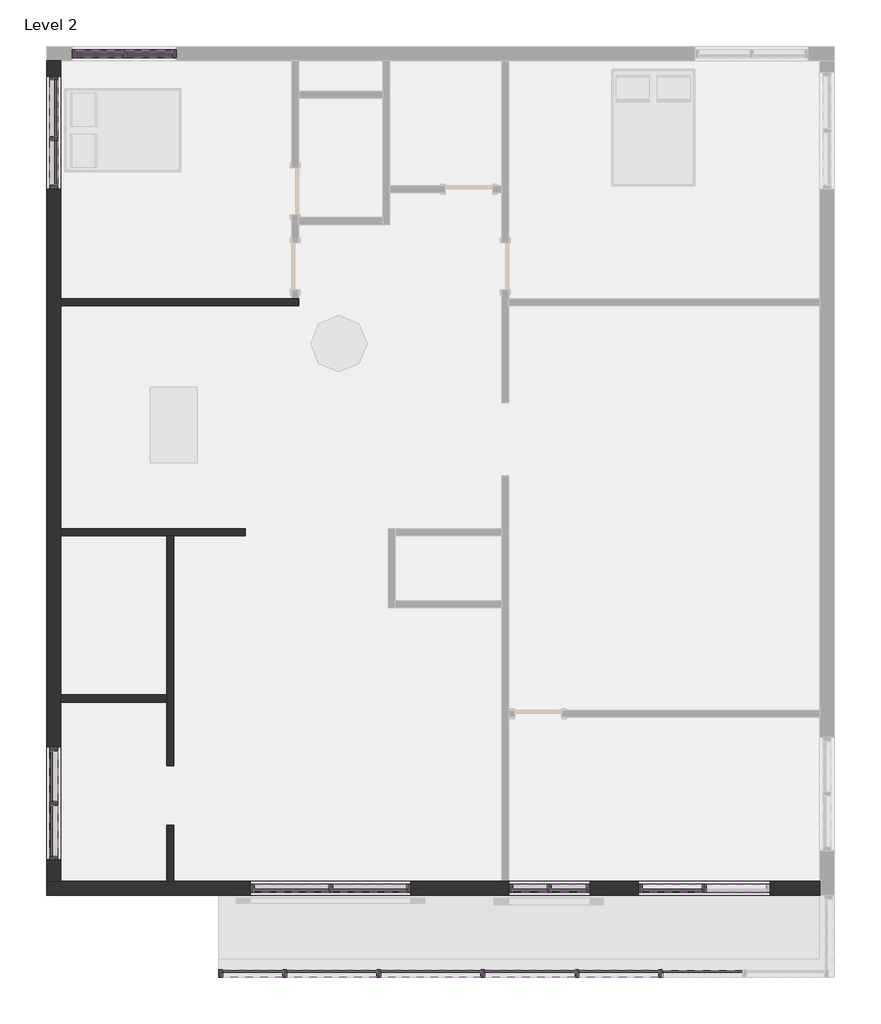
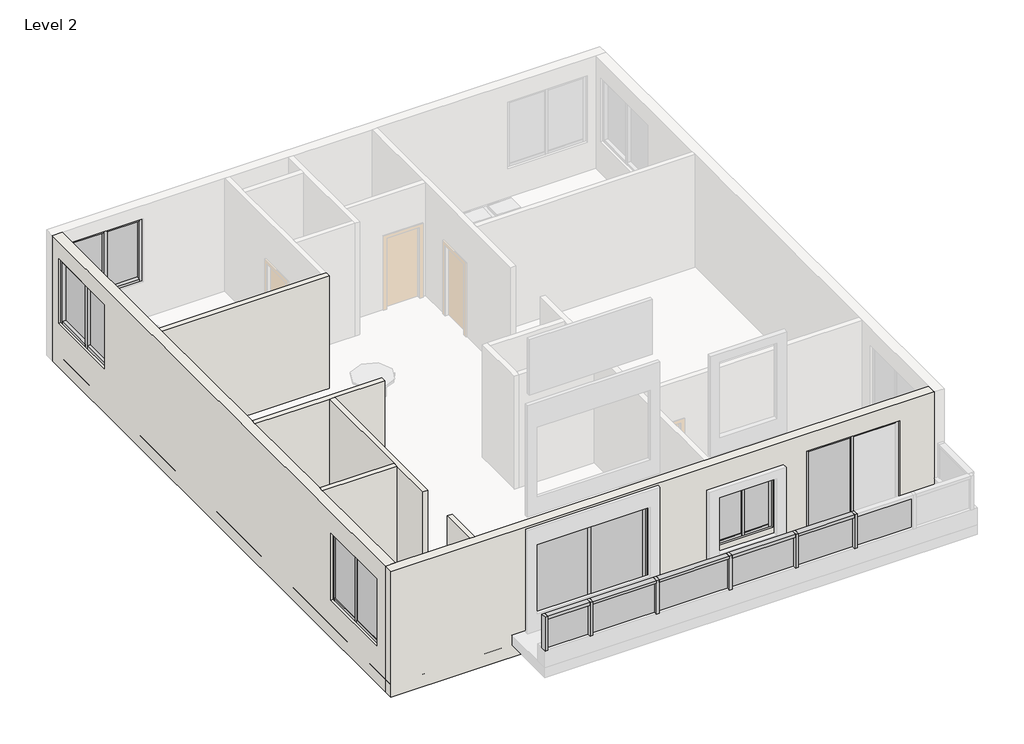
# One storey, part 1 of 2: 50 members, 17 plates, 7 walls.
"""IFC4 building model written with IfcOpenShell, lengths in millimetres."""

from ifc_helpers import new_model, si_unit, frame, origin, place, context, project, spatial, polyline, outline, extrude, faceted_brep, transform, mapped, element, save
from components import member_c17f1be2, member_3a0a7659, member_bb9b20bf, member_f3ef6fbd, member_e04b046a, member_80dcf73b, member_7007ad49, member_ff82125d, member_0ab19f0c, member_973bd760, member_801a2072, member_8e397d51, member_8dd6731c, member_87553b7f, member_e9c7f4a4, member_3112dcca, member_8a344535, member_99d3517c, member_dae9f1c3, member_4a1dde21, member_f7075cef, member_bf3bc0fd, member_d7462ea5, member_8ac64e86, system_panel_glazed_b08c4d22, system_panel_glazed_affe7bbf, system_panel_glazed_9eaa7c8f, system_panel_glazed_b4a21602, system_panel_glazed_4e5a3e53, system_panel_glazed_c585f582, system_panel_glazed_a27b9eb0, system_panel_glazed_060269ed, system_panel_glazed_0d05c03e, system_panel_glazed_4dc74c46, system_panel_glazed_e22b6634

model = new_model("IFC4")

# Units and contexts
model_context = context("Model", 3, world=origin())
ifc_project = project(units=[si_unit("LENGTHUNIT", "METRE", prefix="MILLI")], contexts=[model_context])

# Site, building, storey
site = spatial("IfcSite", under=ifc_project)
building = spatial("IfcBuilding", under=site)
storey = spatial("IfcBuildingStorey", under=building, Name="Level 2", Elevation=3048.0)

# Members
placement = place(None, origin())
member_shape = member_c17f1be2(model_context)
element("IfcMember", 1, ObjectType="Rectangular Mullion : 2.5\" x 5\" rectangular", at=placement, inside=storey, context=model_context, shape_type="MappedRepresentation", body=[
    mapped(member_shape, transform((-18883.3195233, -12680.6252569, 5586.6479842), x_axis=(0.0, 0.0, 1.0), y_axis=(1.0, 0.0, 0.0), z_axis=(0.0, 1.0, 0.0))),
])
element("IfcMember", 2, ObjectType="Rectangular Mullion : 2.5\" x 5\" rectangular", at=placement, inside=storey, context=model_context, shape_type="MappedRepresentation", body=[
    mapped(member_shape, transform((-18883.3195233, -11797.9752569, 5586.6479842), x_axis=(0.0, 0.0, 1.0), y_axis=(1.0, 0.0, 0.0), z_axis=(0.0, 1.0, 0.0))),
])
element("IfcMember", 3, ObjectType="Rectangular Mullion : 2.5\" x 5\" rectangular", at=placement, inside=storey, context=model_context, shape_type="MappedRepresentation", body=[
    mapped(member_shape, transform((-18883.3195233, -12617.1252569, 3956.7332675), x_axis=(0.0, 0.0, -1.0), y_axis=(1.0, 0.0, 0.0), z_axis=(0.0, -1.0, 0.0))),
])
element("IfcMember", 4, ObjectType="Rectangular Mullion : 2.5\" x 5\" rectangular", at=placement, inside=storey, context=model_context, shape_type="MappedRepresentation", body=[
    mapped(member_shape, transform((-18883.3195233, -13499.7752569, 3956.7332675), x_axis=(0.0, 0.0, -1.0), y_axis=(1.0, 0.0, 0.0), z_axis=(0.0, -1.0, 0.0))),
])
member_2_shape = member_3a0a7659(model_context)
element("IfcMember", 5, ObjectType="Rectangular Mullion : 2.5\" x 5\" rectangular", at=placement, inside=storey, context=model_context, shape_type="MappedRepresentation", body=[
    mapped(member_2_shape, transform((-17772.0695233, -533.0752569, 5767.2358325), x_axis=(0.0, 0.0, 1.0), y_axis=(0.0, -1.0, 0.0), z_axis=(1.0, 0.0, 0.0))),
])
element("IfcMember", 6, ObjectType="Rectangular Mullion : 2.5\" x 5\" rectangular", at=placement, inside=storey, context=model_context, shape_type="MappedRepresentation", body=[
    mapped(member_2_shape, transform((-16965.6195233, -533.0752569, 5767.2358325), x_axis=(0.0, 0.0, 1.0), y_axis=(0.0, -1.0, 0.0), z_axis=(1.0, 0.0, 0.0))),
])
element("IfcMember", 7, ObjectType="Rectangular Mullion : 2.5\" x 5\" rectangular", at=placement, inside=storey, context=model_context, shape_type="MappedRepresentation", body=[
    mapped(member_2_shape, transform((-17708.5695233, -533.0752569, 4232.1728983), x_axis=(0.0, 0.0, -1.0), y_axis=(0.0, -1.0, 0.0), z_axis=(-1.0, 0.0, 0.0))),
])
element("IfcMember", 8, ObjectType="Rectangular Mullion : 2.5\" x 5\" rectangular", at=placement, inside=storey, context=model_context, shape_type="MappedRepresentation", body=[
    mapped(member_2_shape, transform((-18515.0195233, -533.0752569, 4232.1728983), x_axis=(0.0, 0.0, -1.0), y_axis=(0.0, -1.0, 0.0), z_axis=(-1.0, 0.0, 0.0))),
])
member_3_shape = member_bb9b20bf(model_context)
element("IfcMember", 9, ObjectType="Rectangular Mullion : 2.5\" x 5\" rectangular", at=placement, inside=storey, context=model_context, shape_type="MappedRepresentation", body=[
    mapped(member_3_shape, transform((-17740.3195233, -533.0752569, 4232.1728983), x_axis=(1.0, 0.0, 0.0), y_axis=(0.0, -1.0, 0.0), z_axis=(0.0, 0.0, -1.0))),
])
member_4_shape = member_f3ef6fbd(model_context)
element("IfcMember", 10, ObjectType="Rectangular Mullion : 2.5\" x 5\" rectangular", at=placement, inside=storey, context=model_context, shape_type="MappedRepresentation", body=[
    mapped(member_4_shape, transform((-18578.5195233, -533.0752569, 5767.2358325), x_axis=(-1.0, 0.0, 0.0), y_axis=(0.0, -1.0, 0.0), z_axis=(0.0, 0.0, 1.0))),
])
element("IfcMember", 11, ObjectType="Rectangular Mullion : 2.5\" x 5\" rectangular", at=placement, inside=storey, context=model_context, shape_type="MappedRepresentation", body=[
    mapped(member_4_shape, transform((-16902.1195233, -533.0752569, 4232.1728983), x_axis=(1.0, 0.0, 0.0), y_axis=(0.0, -1.0, 0.0), z_axis=(0.0, 0.0, -1.0))),
])
member_5_shape = member_e04b046a(model_context)
element("IfcMember", 12, ObjectType="Rectangular Mullion : 2.5\" x 5\" rectangular", at=placement, inside=storey, context=model_context, shape_type="MappedRepresentation", body=[
    mapped(member_5_shape, transform((-18883.3195233, -12648.8752569, 3956.7332675), x_axis=(0.0, 1.0, 0.0), y_axis=(1.0, 0.0, 0.0), z_axis=(0.0, 0.0, -1.0))),
])
member_6_shape = member_80dcf73b(model_context)
element("IfcMember", 13, ObjectType="Rectangular Mullion : 2.5\" x 5\" rectangular", at=placement, inside=storey, context=model_context, shape_type="MappedRepresentation", body=[
    mapped(member_6_shape, transform((-18883.3195233, -13563.2752569, 5586.6479842), x_axis=(0.0, -1.0, 0.0), y_axis=(1.0, 0.0, 0.0), z_axis=(0.0, 0.0, 1.0))),
])
element("IfcMember", 14, ObjectType="Rectangular Mullion : 2.5\" x 5\" rectangular", at=placement, inside=storey, context=model_context, shape_type="MappedRepresentation", body=[
    mapped(member_6_shape, transform((-18883.3195233, -11734.4752569, 3956.7332675), x_axis=(0.0, 1.0, 0.0), y_axis=(1.0, 0.0, 0.0), z_axis=(0.0, 0.0, -1.0))),
])
member_7_shape = member_7007ad49(model_context)
element("IfcMember", 15, ObjectType="Rectangular Mullion : 2.5\" x 5\" rectangular", at=placement, inside=storey, context=model_context, shape_type="MappedRepresentation", body=[
    mapped(member_7_shape, transform((-18883.3195233, -2660.3252569, 5675.9534483), x_axis=(0.0, 0.0, 1.0), y_axis=(-1.0, 0.0, 0.0), z_axis=(0.0, -1.0, 0.0))),
])
member_8_shape = member_ff82125d(model_context)
element("IfcMember", 16, ObjectType="Rectangular Mullion : 2.5\" x 5\" rectangular", at=placement, inside=storey, context=model_context, shape_type="MappedRepresentation", body=[
    mapped(member_8_shape, transform((-18883.3195233, -1879.2752569, 5675.9534483), x_axis=(0.0, 0.0, 1.0), y_axis=(-1.0, 0.0, 0.0), z_axis=(0.0, -1.0, 0.0))),
])
member_9_shape = member_0ab19f0c(model_context)
element("IfcMember", 17, ObjectType="Rectangular Mullion : 2.5\" x 5\" rectangular", at=placement, inside=storey, context=model_context, shape_type="MappedRepresentation", body=[
    mapped(member_9_shape, transform((-18883.3195233, -1911.0252569, 4115.0021153), x_axis=(0.0, -1.0, 0.0), y_axis=(-1.0, 0.0, 0.0), z_axis=(0.0, 0.0, -1.0))),
])
element("IfcMember", 18, ObjectType="Rectangular Mullion : 2.5\" x 5\" rectangular", at=placement, inside=storey, context=model_context, shape_type="MappedRepresentation", body=[
    mapped(member_7_shape, transform((-18883.3195233, -1942.7752569, 4115.0021153), x_axis=(0.0, 0.0, -1.0), y_axis=(-1.0, 0.0, 0.0), z_axis=(0.0, 1.0, 0.0))),
])
element("IfcMember", 19, ObjectType="Rectangular Mullion : 2.5\" x 5\" rectangular", at=placement, inside=storey, context=model_context, shape_type="MappedRepresentation", body=[
    mapped(member_8_shape, transform((-18883.3195233, -958.5252569, 4115.0021153), x_axis=(0.0, 0.0, -1.0), y_axis=(-1.0, 0.0, 0.0), z_axis=(0.0, 1.0, 0.0))),
])
member_10_shape = member_973bd760(model_context)
element("IfcMember", 20, ObjectType="Rectangular Mullion : 2.5\" x 5\" rectangular", at=placement, inside=storey, context=model_context, shape_type="MappedRepresentation", body=[
    mapped(member_10_shape, transform((-18883.3195233, -2723.8252569, 4115.0021153), x_axis=(0.0, -1.0, 0.0), y_axis=(-1.0, 0.0, 0.0), z_axis=(0.0, 0.0, -1.0))),
])
element("IfcMember", 21, ObjectType="Rectangular Mullion : 2.5\" x 5\" rectangular", at=placement, inside=storey, context=model_context, shape_type="MappedRepresentation", body=[
    mapped(member_10_shape, transform((-18883.3195233, -895.0252569, 5675.9534483), x_axis=(0.0, 1.0, 0.0), y_axis=(-1.0, 0.0, 0.0), z_axis=(0.0, 0.0, 1.0))),
])
member_11_shape = member_801a2072(model_context)
element("IfcMember", 22, ObjectType="Rectangular Mullion : 2.5\" x 5\" rectangular", at=placement, inside=storey, context=model_context, shape_type="MappedRepresentation", body=[
    mapped(member_11_shape, transform((-8335.9695233, -14020.4752569, 5682.139627), x_axis=(0.0, 0.0, 1.0), y_axis=(0.0, 1.0, 0.0), z_axis=(-1.0, 0.0, 0.0))),
])
element("IfcMember", 23, ObjectType="Rectangular Mullion : 2.5\" x 5\" rectangular", at=placement, inside=storey, context=model_context, shape_type="MappedRepresentation", body=[
    mapped(member_11_shape, transform((-9371.0195233, -14020.4752569, 5682.139627), x_axis=(0.0, 0.0, 1.0), y_axis=(0.0, 1.0, 0.0), z_axis=(-1.0, 0.0, 0.0))),
])
element("IfcMember", 24, ObjectType="Rectangular Mullion : 2.5\" x 5\" rectangular", at=placement, inside=storey, context=model_context, shape_type="MappedRepresentation", body=[
    mapped(member_11_shape, transform((-15182.1712454, -15398.1130528, 4822.8286641), x_axis=(0.0, 0.0, 1.0), y_axis=(0.0, -1.0, 0.0), z_axis=(1.0, 0.0, 0.0))),
])
member_12_shape = member_8e397d51(model_context)
element("IfcMember", 25, ObjectType="Rectangular Mullion : 2.5\" x 5\" rectangular", at=placement, inside=storey, context=model_context, shape_type="MappedRepresentation", body=[
    mapped(member_12_shape, transform((-10841.0445233, -14020.4752569, 5377.8228134), x_axis=(0.0, 0.0, 1.0), y_axis=(0.0, 1.0, 0.0), z_axis=(-1.0, 0.0, 0.0))),
])
element("IfcMember", 26, ObjectType="Rectangular Mullion : 2.5\" x 5\" rectangular", at=placement, inside=storey, context=model_context, shape_type="MappedRepresentation", body=[
    mapped(member_12_shape, transform((-11466.5195233, -14020.4752569, 5377.8228134), x_axis=(0.0, 0.0, 1.0), y_axis=(0.0, 1.0, 0.0), z_axis=(-1.0, 0.0, 0.0))),
])
member_13_shape = member_8dd6731c(model_context)
element("IfcMember", 27, ObjectType="Rectangular Mullion : 2.5\" x 5\" rectangular", at=placement, inside=storey, context=model_context, shape_type="MappedRepresentation", body=[
    mapped(member_13_shape, transform((-10872.7945233, -14020.4752569, 4104.4168129), x_axis=(-1.0, 0.0, 0.0), y_axis=(0.0, 1.0, 0.0), z_axis=(0.0, 0.0, -1.0))),
])
element("IfcMember", 28, ObjectType="Rectangular Mullion : 2.5\" x 5\" rectangular", at=placement, inside=storey, context=model_context, shape_type="MappedRepresentation", body=[
    mapped(member_12_shape, transform((-10904.5445233, -14020.4752569, 4104.4168129), x_axis=(0.0, 0.0, -1.0), y_axis=(0.0, 1.0, 0.0), z_axis=(1.0, 0.0, 0.0))),
])
element("IfcMember", 29, ObjectType="Rectangular Mullion : 2.5\" x 5\" rectangular", at=placement, inside=storey, context=model_context, shape_type="MappedRepresentation", body=[
    mapped(member_12_shape, transform((-10279.0695233, -14020.4752569, 4104.4168129), x_axis=(0.0, 0.0, -1.0), y_axis=(0.0, 1.0, 0.0), z_axis=(1.0, 0.0, 0.0))),
])
member_14_shape = member_87553b7f(model_context)
element("IfcMember", 30, ObjectType="Rectangular Mullion : 2.5\" x 5\" rectangular", at=placement, inside=storey, context=model_context, shape_type="MappedRepresentation", body=[
    mapped(member_14_shape, transform((-10215.5695233, -14020.4752569, 5377.8228134), x_axis=(1.0, 0.0, 0.0), y_axis=(0.0, 1.0, 0.0), z_axis=(0.0, 0.0, 1.0))),
])
element("IfcMember", 31, ObjectType="Rectangular Mullion : 2.5\" x 5\" rectangular", at=placement, inside=storey, context=model_context, shape_type="MappedRepresentation", body=[
    mapped(member_14_shape, transform((-11530.0195233, -14020.4752569, 4104.4168129), x_axis=(-1.0, 0.0, 0.0), y_axis=(0.0, 1.0, 0.0), z_axis=(0.0, 0.0, -1.0))),
])
member_15_shape = member_e9c7f4a4(model_context)
element("IfcMember", 32, ObjectType="Rectangular Mullion : 2.5\" x 5\" rectangular", at=placement, inside=storey, context=model_context, shape_type="MappedRepresentation", body=[
    mapped(member_15_shape, transform((-14374.8195233, -14020.4752569, 5678.6814593), x_axis=(0.0, 0.0, 1.0), y_axis=(0.0, 1.0, 0.0), z_axis=(-1.0, 0.0, 0.0))),
])
element("IfcMember", 33, ObjectType="Rectangular Mullion : 2.5\" x 5\" rectangular", at=placement, inside=storey, context=model_context, shape_type="MappedRepresentation", body=[
    mapped(member_15_shape, transform((-15638.4695233, -14020.4752569, 5678.6814593), x_axis=(0.0, 0.0, 1.0), y_axis=(0.0, 1.0, 0.0), z_axis=(-1.0, 0.0, 0.0))),
])
element("IfcMember", 34, ObjectType="Rectangular Mullion : 2.5\" x 5\" rectangular", at=placement, inside=storey, context=model_context, shape_type="MappedRepresentation", body=[
    mapped(member_15_shape, transform((-14438.3195233, -14020.4752569, 3707.8481759), x_axis=(0.0, 0.0, -1.0), y_axis=(0.0, 1.0, 0.0), z_axis=(1.0, 0.0, 0.0))),
])
element("IfcMember", 35, ObjectType="Rectangular Mullion : 2.5\" x 5\" rectangular", at=placement, inside=storey, context=model_context, shape_type="MappedRepresentation", body=[
    mapped(member_15_shape, transform((-13174.6695233, -14020.4752569, 3707.8481759), x_axis=(0.0, 0.0, -1.0), y_axis=(0.0, 1.0, 0.0), z_axis=(1.0, 0.0, 0.0))),
])
member_16_shape = member_3112dcca(model_context)
element("IfcMember", 36, ObjectType="Rectangular Mullion : 2.5\" x 5\" rectangular", at=placement, inside=storey, context=model_context, shape_type="MappedRepresentation", body=[
    mapped(member_16_shape, transform((-14406.5695233, -14020.4752569, 3707.8481759), x_axis=(-1.0, 0.0, 0.0), y_axis=(0.0, 1.0, 0.0), z_axis=(0.0, 0.0, -1.0))),
])
member_17_shape = member_8a344535(model_context)
element("IfcMember", 37, ObjectType="Rectangular Mullion : 2.5\" x 5\" rectangular", at=placement, inside=storey, context=model_context, shape_type="MappedRepresentation", body=[
    mapped(member_17_shape, transform((-13111.1695233, -14020.4752569, 5678.6814593), x_axis=(1.0, 0.0, 0.0), y_axis=(0.0, 1.0, 0.0), z_axis=(0.0, 0.0, 1.0))),
])
element("IfcMember", 38, ObjectType="Rectangular Mullion : 2.5\" x 5\" rectangular", at=placement, inside=storey, context=model_context, shape_type="MappedRepresentation", body=[
    mapped(member_17_shape, transform((-15701.9695233, -14020.4752569, 3707.8481759), x_axis=(-1.0, 0.0, 0.0), y_axis=(0.0, 1.0, 0.0), z_axis=(0.0, 0.0, -1.0))),
])
member_18_shape = member_99d3517c(model_context)
element("IfcMember", 39, ObjectType="Rectangular Mullion : 2.5\" x 5\" rectangular", at=placement, inside=storey, context=model_context, shape_type="MappedRepresentation", body=[
    mapped(member_18_shape, transform((-8367.7195233, -14020.4752569, 3693.4399111), x_axis=(-1.0, 0.0, 0.0), y_axis=(0.0, 1.0, 0.0), z_axis=(0.0, 0.0, -1.0))),
])
member_19_shape = member_dae9f1c3(model_context)
element("IfcMember", 40, ObjectType="Rectangular Mullion : 2.5\" x 5\" rectangular", at=placement, inside=storey, context=model_context, shape_type="MappedRepresentation", body=[
    mapped(member_19_shape, transform((-9434.5195233, -14020.4752569, 3693.4399111), x_axis=(-1.0, 0.0, 0.0), y_axis=(0.0, 1.0, 0.0), z_axis=(0.0, 0.0, -1.0))),
])
member_20_shape = member_4a1dde21(model_context)
element("IfcMember", 41, ObjectType="Rectangular Mullion : 2.5\" x 5\" rectangular", at=placement, inside=storey, context=model_context, shape_type="MappedRepresentation", body=[
    mapped(member_20_shape, transform((-10457.7712454, -15398.1130528, 4822.8286641), x_axis=(0.0, 0.0, 1.0), y_axis=(0.0, -1.0, 0.0), z_axis=(1.0, 0.0, 0.0))),
])
element("IfcMember", 42, ObjectType="Rectangular Mullion : 2.5\" x 5\" rectangular", at=placement, inside=storey, context=model_context, shape_type="MappedRepresentation", body=[
    mapped(member_20_shape, transform((-13658.1712454, -15398.1130528, 4822.8286641), x_axis=(0.0, 0.0, 1.0), y_axis=(0.0, -1.0, 0.0), z_axis=(1.0, 0.0, 0.0))),
])
member_21_shape = member_f7075cef(model_context)
element("IfcMember", 43, ObjectType="Rectangular Mullion : 2.5\" x 5\" rectangular", at=placement, inside=storey, context=model_context, shape_type="MappedRepresentation", body=[
    mapped(member_21_shape, transform((-11981.7712454, -15398.1130528, 4822.8286641), x_axis=(0.0, 0.0, 1.0), y_axis=(0.0, -1.0, 0.0), z_axis=(1.0, 0.0, 0.0))),
])
member_22_shape = member_bf3bc0fd(model_context)
element("IfcMember", 44, ObjectType="Rectangular Mullion : 2.5\" x 5\" rectangular", at=placement, inside=storey, context=model_context, shape_type="MappedRepresentation", body=[
    mapped(member_22_shape, transform((-9103.1045788, -15398.1130528, 4822.8286641), x_axis=(0.0, 0.0, 1.0), y_axis=(0.0, -1.0, 0.0), z_axis=(1.0, 0.0, 0.0))),
])
member_23_shape = member_d7462ea5(model_context)
element("IfcMember", 45, ObjectType="Rectangular Mullion : 2.5\" x 5\" rectangular", at=placement, inside=storey, context=model_context, shape_type="MappedRepresentation", body=[
    mapped(member_23_shape, transform((-15150.4212454, -15398.1130528, 4001.8016497), x_axis=(1.0, 0.0, 0.0), y_axis=(0.0, -1.0, 0.0), z_axis=(0.0, 0.0, -1.0))),
])
element("IfcMember", 46, ObjectType="Rectangular Mullion : 2.5\" x 5\" rectangular", at=placement, inside=storey, context=model_context, shape_type="MappedRepresentation", body=[
    mapped(member_23_shape, transform((-13626.4212454, -15398.1130528, 4001.8016497), x_axis=(1.0, 0.0, 0.0), y_axis=(0.0, -1.0, 0.0), z_axis=(0.0, 0.0, -1.0))),
])
element("IfcMember", 47, ObjectType="Rectangular Mullion : 2.5\" x 5\" rectangular", at=placement, inside=storey, context=model_context, shape_type="MappedRepresentation", body=[
    mapped(member_23_shape, transform((-11950.0212454, -15398.1130528, 4001.8016497), x_axis=(1.0, 0.0, 0.0), y_axis=(0.0, -1.0, 0.0), z_axis=(0.0, 0.0, -1.0))),
])
element("IfcMember", 48, ObjectType="Rectangular Mullion : 2.5\" x 5\" rectangular", at=placement, inside=storey, context=model_context, shape_type="MappedRepresentation", body=[
    mapped(member_23_shape, transform((-10426.0212454, -15398.1130528, 4001.8016497), x_axis=(1.0, 0.0, 0.0), y_axis=(0.0, -1.0, 0.0), z_axis=(0.0, 0.0, -1.0))),
])
element("IfcMember", 49, ObjectType="Rectangular Mullion : 2.5\" x 5\" rectangular", at=placement, inside=storey, context=model_context, shape_type="MappedRepresentation", body=[
    mapped(member_23_shape, transform((-9071.3545788, -15398.1130528, 4001.8016497), x_axis=(1.0, 0.0, 0.0), y_axis=(0.0, -1.0, 0.0), z_axis=(0.0, 0.0, -1.0))),
])
member_24_shape = member_8ac64e86(model_context)
element("IfcMember", 50, ObjectType="Rectangular Mullion : 2.5\" x 5\" rectangular", at=placement, inside=storey, context=model_context, shape_type="MappedRepresentation", body=[
    mapped(member_24_shape, transform((-16217.2212454, -15398.1130528, 4822.8286641), x_axis=(-1.0, 0.0, 0.0), y_axis=(0.0, -1.0, 0.0), z_axis=(0.0, 0.0, 1.0))),
])

# Plates
system_panel_glazed_shape = system_panel_glazed_b08c4d22(model_context)
element("IfcPlate", 51, ObjectType="System Panel : Glazed", at=placement, inside=storey, context=model_context, shape_type="MappedRepresentation", body=[
    mapped(system_panel_glazed_shape, transform((-18143.5445233, -533.0752569, 4295.6728983), x_axis=(1.0, 0.0, 0.0), y_axis=(0.0, 1.0, 0.0), z_axis=(0.0, 0.0, 1.0))),
])
element("IfcPlate", 52, ObjectType="System Panel : Glazed", at=placement, inside=storey, context=model_context, shape_type="MappedRepresentation", body=[
    mapped(system_panel_glazed_shape, transform((-17337.0945233, -533.0752569, 4295.6728983), x_axis=(1.0, 0.0, 0.0), y_axis=(0.0, 1.0, 0.0), z_axis=(0.0, 0.0, 1.0))),
])
system_panel_glazed_2_shape = system_panel_glazed_affe7bbf(model_context)
element("IfcPlate", 53, ObjectType="System Panel : Glazed", at=placement, inside=storey, context=model_context, shape_type="MappedRepresentation", body=[
    mapped(system_panel_glazed_2_shape, transform((-18883.3195233, -13090.2002569, 4020.2332675), x_axis=(0.0, 1.0, 0.0), y_axis=(-1.0, 0.0, 0.0), z_axis=(0.0, 0.0, 1.0))),
])
element("IfcPlate", 54, ObjectType="System Panel : Glazed", at=placement, inside=storey, context=model_context, shape_type="MappedRepresentation", body=[
    mapped(system_panel_glazed_2_shape, transform((-18883.3195233, -12207.5502569, 4020.2332675), x_axis=(0.0, 1.0, 0.0), y_axis=(-1.0, 0.0, 0.0), z_axis=(0.0, 0.0, 1.0))),
])
system_panel_glazed_3_shape = system_panel_glazed_9eaa7c8f(model_context)
element("IfcPlate", 55, ObjectType="System Panel : Glazed", at=placement, inside=storey, context=model_context, shape_type="MappedRepresentation", body=[
    mapped(system_panel_glazed_3_shape, transform((-18883.3195233, -1418.9002569, 4178.5021153), x_axis=(0.0, -1.0, 0.0), y_axis=(1.0, 0.0, 0.0), z_axis=(0.0, 0.0, 1.0))),
])
system_panel_glazed_4_shape = system_panel_glazed_b4a21602(model_context)
element("IfcPlate", 56, ObjectType="System Panel : Glazed", at=placement, inside=storey, context=model_context, shape_type="MappedRepresentation", body=[
    mapped(system_panel_glazed_4_shape, transform((-18883.3195233, -2301.5502569, 4178.5021153), x_axis=(0.0, -1.0, 0.0), y_axis=(1.0, 0.0, 0.0), z_axis=(0.0, 0.0, 1.0))),
])
system_panel_glazed_5_shape = system_panel_glazed_4e5a3e53(model_context)
element("IfcPlate", 57, ObjectType="System Panel : Glazed", at=placement, inside=storey, context=model_context, shape_type="MappedRepresentation", body=[
    mapped(system_panel_glazed_5_shape, transform((-10560.0570233, -14020.4752569, 4167.9168129), x_axis=(-1.0, 0.0, 0.0), y_axis=(0.0, -1.0, 0.0), z_axis=(0.0, 0.0, 1.0))),
])
element("IfcPlate", 58, ObjectType="System Panel : Glazed", at=placement, inside=storey, context=model_context, shape_type="MappedRepresentation", body=[
    mapped(system_panel_glazed_5_shape, transform((-11185.5320233, -14020.4752569, 4167.9168129), x_axis=(-1.0, 0.0, 0.0), y_axis=(0.0, -1.0, 0.0), z_axis=(0.0, 0.0, 1.0))),
])
system_panel_glazed_6_shape = system_panel_glazed_c585f582(model_context)
element("IfcPlate", 59, ObjectType="System Panel : Glazed", at=placement, inside=storey, context=model_context, shape_type="MappedRepresentation", body=[
    mapped(system_panel_glazed_6_shape, transform((-13774.7445233, -14020.4752569, 3771.3481759), x_axis=(-1.0, 0.0, 0.0), y_axis=(0.0, -1.0, 0.0), z_axis=(0.0, 0.0, 1.0))),
])
element("IfcPlate", 60, ObjectType="System Panel : Glazed", at=placement, inside=storey, context=model_context, shape_type="MappedRepresentation", body=[
    mapped(system_panel_glazed_6_shape, transform((-15038.3945233, -14020.4752569, 3771.3481759), x_axis=(-1.0, 0.0, 0.0), y_axis=(0.0, -1.0, 0.0), z_axis=(0.0, 0.0, 1.0))),
])
system_panel_glazed_7_shape = system_panel_glazed_a27b9eb0(model_context)
element("IfcPlate", 61, ObjectType="System Panel : Glazed", at=placement, inside=storey, context=model_context, shape_type="MappedRepresentation", body=[
    mapped(system_panel_glazed_7_shape, transform((-8885.2445233, -14020.4752569, 3756.9399111), x_axis=(-1.0, 0.0, 0.0), y_axis=(0.0, -1.0, 0.0), z_axis=(0.0, 0.0, 1.0))),
])
system_panel_glazed_8_shape = system_panel_glazed_060269ed(model_context)
element("IfcPlate", 62, ObjectType="System Panel : Glazed", at=placement, inside=storey, context=model_context, shape_type="MappedRepresentation", body=[
    mapped(system_panel_glazed_8_shape, transform((-9748.6879121, -15398.1130528, 4001.8016497), x_axis=(1.0, 0.0, 0.0), y_axis=(0.0, 1.0, 0.0), z_axis=(0.0, 0.0, 1.0))),
])
element("IfcPlate", 63, ObjectType="System Panel : Glazed", at=placement, inside=storey, context=model_context, shape_type="MappedRepresentation", body=[
    mapped(system_panel_glazed_8_shape, transform((-8394.0212454, -15398.1130528, 4001.8016497), x_axis=(1.0, 0.0, 0.0), y_axis=(0.0, 1.0, 0.0), z_axis=(0.0, 0.0, 1.0))),
])
system_panel_glazed_9_shape = system_panel_glazed_0d05c03e(model_context)
element("IfcPlate", 64, ObjectType="System Panel : Glazed", at=placement, inside=storey, context=model_context, shape_type="MappedRepresentation", body=[
    mapped(system_panel_glazed_9_shape, transform((-14388.4212454, -15398.1130528, 4001.8016497), x_axis=(1.0, 0.0, 0.0), y_axis=(0.0, 1.0, 0.0), z_axis=(0.0, 0.0, 1.0))),
])
element("IfcPlate", 65, ObjectType="System Panel : Glazed", at=placement, inside=storey, context=model_context, shape_type="MappedRepresentation", body=[
    mapped(system_panel_glazed_9_shape, transform((-11188.0212454, -15398.1130528, 4001.8016497), x_axis=(1.0, 0.0, 0.0), y_axis=(0.0, 1.0, 0.0), z_axis=(0.0, 0.0, 1.0))),
])
system_panel_glazed_10_shape = system_panel_glazed_4dc74c46(model_context)
element("IfcPlate", 66, ObjectType="System Panel : Glazed", at=placement, inside=storey, context=model_context, shape_type="MappedRepresentation", body=[
    mapped(system_panel_glazed_10_shape, transform((-12788.2212454, -15398.1130528, 4001.8016497), x_axis=(1.0, 0.0, 0.0), y_axis=(0.0, 1.0, 0.0), z_axis=(0.0, 0.0, 1.0))),
])
system_panel_glazed_11_shape = system_panel_glazed_e22b6634(model_context)
element("IfcPlate", 67, ObjectType="System Panel : Glazed", at=placement, inside=storey, context=model_context, shape_type="MappedRepresentation", body=[
    mapped(system_panel_glazed_11_shape, transform((-15667.9462454, -15398.1130528, 4001.8016497), x_axis=(1.0, 0.0, 0.0), y_axis=(0.0, 1.0, 0.0), z_axis=(0.0, 0.0, 1.0))),
])

# Walls
element("IfcWall", 68, ObjectType="4.5\"", at=placement, inside=storey, context=model_context, shape_type="Brep", body=[
    faceted_brep([(-18769.0195233, -4609.7752569, 3048.0), (-14920.9195233, -4609.7752569, 3048.0), (-14920.9195233, -4609.7752569, 6096.0), (-18769.0195233, -4609.7752569, 6096.0), (-18769.0195233, -4495.4752569, 3048.0), (-18769.0195233, -4495.4752569, 6096.0), (-15035.2195233, -4495.4752569, 6096.0), (-14920.9195233, -4495.4752569, 6096.0), (-14920.9195233, -4495.4752569, 3048.0), (-15035.2195233, -4495.4752569, 3048.0)], [[[0, 1, 2, 3]], [[4, 5, 6, 7, 8, 9]], [[1, 0, 4, 9, 8]], [[3, 2, 7, 6, 5]], [[0, 3, 5, 4]], [[2, 1, 8, 7]]]),
])
element("IfcWall", 69, ObjectType="4.5\"", at=placement, inside=storey, context=model_context, shape_type="Brep", body=[
    faceted_brep([(-18769.0195233, -8324.5252569, 3048.0), (-17054.5195233, -8324.5252569, 3048.0), (-16940.2195233, -8324.5252569, 3048.0), (-15784.5195233, -8324.5252569, 3048.0), (-15784.5195233, -8324.5252569, 6096.0), (-16940.2195233, -8324.5252569, 6096.0), (-17054.5195233, -8324.5252569, 6096.0), (-18769.0195233, -8324.5252569, 6096.0), (-18769.0195233, -8210.2252569, 3048.0), (-18769.0195233, -8210.2252569, 6096.0), (-15784.5195233, -8210.2252569, 6096.0), (-15784.5195233, -8210.2252569, 3048.0)], [[[0, 1, 2, 3, 4, 5, 6, 7]], [[8, 9, 10, 11]], [[3, 2, 1, 0, 8, 11]], [[4, 3, 11, 10]], [[7, 6, 5, 4, 10, 9]], [[0, 7, 9, 8]]]),
])
element("IfcWall", 70, ObjectType="4.5\"", at=placement, inside=storey, context=model_context, shape_type="Brep", body=[
    faceted_brep([(-17054.5195233, -8324.5252569, 3048.0), (-17054.5195233, -10896.2752569, 3048.0), (-17054.5195233, -11010.5752569, 3048.0), (-17054.5195233, -12039.2752569, 3048.0), (-17054.5195233, -12039.2752569, 6096.0), (-17054.5195233, -11010.5752569, 6096.0), (-17054.5195233, -10896.2752569, 6096.0), (-17054.5195233, -8324.5252569, 6096.0), (-16940.2195233, -8324.5252569, 3048.0), (-16940.2195233, -8324.5252569, 6096.0), (-16940.2195233, -12039.2752569, 6096.0), (-16940.2195233, -12039.2752569, 3048.0)], [[[0, 1, 2, 3, 4, 5, 6, 7]], [[8, 9, 10, 11]], [[3, 2, 1, 0, 8, 11]], [[4, 3, 11, 10]], [[7, 6, 5, 4, 10, 9]], [[0, 7, 9, 8]]]),
])
element("IfcWall", 71, ObjectType="4.5\"", at=placement, inside=storey, context=model_context, shape_type="SweptSolid", body=[
    extrude(outline(polyline([(-17054.5195233, -11010.5752569), (-18769.0195233, -11010.5752569), (-18769.0195233, -10896.2752569), (-17054.5195233, -10896.2752569), (-17054.5195233, -11010.5752569)])), frame((0.0, 0.0, 3048.0), z_axis=(0.0, 0.0, 1.0), x_axis=(1.0, 0.0, 0.0)), (0.0, 0.0, 1.0), 3048.0),
])
element("IfcWall", 72, ObjectType="4.5\"", at=placement, inside=storey, context=model_context, shape_type="SweptSolid", body=[
    extrude(outline(polyline([(-16940.2195233, -13004.4752569), (-16940.2195233, -13906.1752569), (-17054.5195233, -13906.1752569), (-17054.5195233, -13004.4752569), (-16940.2195233, -13004.4752569)])), frame((0.0, 0.0, 3048.0), z_axis=(0.0, 0.0, 1.0), x_axis=(1.0, 0.0, 0.0)), (0.0, 0.0, 1.0), 3048.0),
])
element("IfcWall", 73, ObjectType="9\"", at=placement, inside=storey, context=model_context, shape_type="Brep", body=[
    faceted_brep([(-6500.8195233, -13906.1752569, 3048.0), (-11530.0195233, -13906.1752569, 3048.0), (-11644.3195233, -13906.1752569, 3048.0), (-16940.2195233, -13906.1752569, 3048.0), (-17054.5195233, -13906.1752569, 3048.0), (-18769.0195233, -13906.1752569, 3048.0), (-18997.6195233, -13906.1752569, 3048.0), (-18997.6195233, -13906.1752569, 6096.0), (-18769.0195233, -13906.1752569, 6096.0), (-17054.5195233, -13906.1752569, 6096.0), (-16940.2195233, -13906.1752569, 6096.0), (-11644.3195233, -13906.1752569, 6096.0), (-11530.0195233, -13906.1752569, 6096.0), (-6500.8195233, -13906.1752569, 6096.0), (-7300.9195233, -13906.1752569, 3693.4399111), (-7300.9195233, -13906.1752569, 5682.139627), (-9434.5195233, -13906.1752569, 5682.139627), (-9434.5195233, -13906.1752569, 3693.4399111), (-10215.5695233, -13906.1752569, 4104.4168129), (-10215.5695233, -13906.1752569, 5377.8228134), (-11530.0195233, -13906.1752569, 5377.8228134), (-11530.0195233, -13906.1752569, 4104.4168129), (-13111.1695233, -13906.1752569, 3707.8481759), (-13111.1695233, -13906.1752569, 5678.6814593), (-15701.9695233, -13906.1752569, 5678.6814593), (-15701.9695233, -13906.1752569, 3707.8481759), (-18997.6195233, -14134.7752569, 3048.0), (-6500.8195233, -14134.7752569, 3048.0), (-6500.8195233, -14134.7752569, 6096.0), (-18997.6195233, -14134.7752569, 6096.0), (-7300.9195233, -14134.7752569, 5682.139627), (-7300.9195233, -14134.7752569, 3693.4399111), (-9434.5195233, -14134.7752569, 3693.4399111), (-9434.5195233, -14134.7752569, 5682.139627), (-10215.5695233, -14134.7752569, 5377.8228134), (-10215.5695233, -14134.7752569, 4104.4168129), (-11530.0195233, -14134.7752569, 4104.4168129), (-11530.0195233, -14134.7752569, 5377.8228134), (-13111.1695233, -14134.7752569, 5678.6814593), (-13111.1695233, -14134.7752569, 3707.8481759), (-15701.9695233, -14134.7752569, 3707.8481759), (-15701.9695233, -14134.7752569, 5678.6814593)], [[[0, 1, 2, 3, 4, 5, 6, 7, 8, 9, 10, 11, 12, 13], [14, 15, 16, 17], [18, 19, 20, 21], [22, 23, 24, 25]], [[26, 27, 28, 29], [30, 31, 32, 33], [34, 35, 36, 37], [38, 39, 40, 41]], [[6, 5, 4, 3, 2, 1, 0, 27, 26]], [[13, 12, 11, 10, 9, 8, 7, 29, 28]], [[7, 6, 26, 29]], [[0, 13, 28, 27]], [[30, 15, 14, 31]], [[15, 30, 33, 16]], [[16, 33, 32, 17]], [[31, 14, 17, 32]], [[18, 35, 34, 19]], [[19, 34, 37, 20]], [[36, 21, 20, 37]], [[35, 18, 21, 36]], [[22, 39, 38, 23]], [[23, 38, 41, 24]], [[24, 41, 40, 25]], [[39, 22, 25, 40]]]),
])
element("IfcWall", 74, ObjectType="9\"", at=placement, inside=storey, context=model_context, shape_type="Brep", body=[
    faceted_brep([(-18769.0195233, -13906.1752569, 3048.0), (-18769.0195233, -11010.5752569, 3048.0), (-18769.0195233, -10896.2752569, 3048.0), (-18769.0195233, -8324.5252569, 3048.0), (-18769.0195233, -8210.2252569, 3048.0), (-18769.0195233, -4609.7752569, 3048.0), (-18769.0195233, -4495.4752569, 3048.0), (-18769.0195233, -647.3752569, 3048.0), (-18769.0195233, -647.3752569, 6096.0), (-18769.0195233, -4495.4752569, 6096.0), (-18769.0195233, -4609.7752569, 6096.0), (-18769.0195233, -8210.2252569, 6096.0), (-18769.0195233, -8324.5252569, 6096.0), (-18769.0195233, -10896.2752569, 6096.0), (-18769.0195233, -11010.5752569, 6096.0), (-18769.0195233, -13906.1752569, 6096.0), (-18769.0195233, -895.0252569, 5675.9534483), (-18769.0195233, -895.0252569, 4115.0021153), (-18769.0195233, -2723.8252569, 4115.0021153), (-18769.0195233, -2723.8252569, 5675.9534483), (-18769.0195233, -13563.2752569, 3956.7332675), (-18769.0195233, -13563.2752569, 5586.6479842), (-18769.0195233, -11734.4752569, 5586.6479842), (-18769.0195233, -11734.4752569, 3956.7332675), (-18997.6195233, -647.3752569, 3048.0), (-18997.6195233, -13906.1752569, 3048.0), (-18997.6195233, -13906.1752569, 6096.0), (-18997.6195233, -647.3752569, 6096.0), (-18997.6195233, -895.0252569, 4115.0021153), (-18997.6195233, -895.0252569, 5675.9534483), (-18997.6195233, -2723.8252569, 5675.9534483), (-18997.6195233, -2723.8252569, 4115.0021153), (-18997.6195233, -13563.2752569, 5586.6479842), (-18997.6195233, -13563.2752569, 3956.7332675), (-18997.6195233, -11734.4752569, 3956.7332675), (-18997.6195233, -11734.4752569, 5586.6479842)], [[[0, 1, 2, 3, 4, 5, 6, 7, 8, 9, 10, 11, 12, 13, 14, 15], [16, 17, 18, 19], [20, 21, 22, 23]], [[24, 25, 26, 27], [28, 29, 30, 31], [32, 33, 34, 35]], [[7, 6, 5, 4, 3, 2, 1, 0, 25, 24]], [[15, 14, 13, 12, 11, 10, 9, 8, 27, 26]], [[8, 7, 24, 27]], [[0, 15, 26, 25]], [[28, 17, 16, 29]], [[29, 16, 19, 30]], [[30, 19, 18, 31]], [[17, 28, 31, 18]], [[20, 33, 32, 21]], [[21, 32, 35, 22]], [[34, 23, 22, 35]], [[33, 20, 23, 34]]]),
])

save(model, "model.ifc")

# Revit data of these elements
# Type "Rectangular Mullion : 2.5\" x 5\" rectangular"
#   built-in parameter 1007304 = 0.416667 (stored number, unit not read)
#   built-in parameter 1007301 = 0.104167 (stored number, unit not read)
#   built-in parameter 1007300 = 0.104167 (stored number, unit not read)
# Type "System Panel : Glazed"
#   Construction Type Id = "GSP4R"
#   Analytic Construction = "1/8 in Pilkington single glazing"
#   Visual Light Transmittance = 0.9
#   Solar Heat Gain Coefficient = 0.86
#   Heat Transfer Coefficient (U) = 1.18115 BTU/(h·ft²·°F)
#   Define Thermal Properties by = 1
# Type "4.5\""
#   Assembly Code = "B2010"
#   Layers, outside or top first: 0' - 4 1/2" no material (function 1)
# Type "9\""
#   Assembly Code = "B2010"
#   Layers, outside or top first: 0' - 9" no material (function 1)
# Elements 1, 2, 3, 4, 5, 6, 7, 8, 9, 10, 11, 12, 13, 14, 15, 16, 17, 18, 19, 20, 21, 22, 23, 24, 25, 26, 27, 28, 29, 30, 31, 32, 33, 34, 35, 36, 37, 38, 39, 40, 41, 42, 43, 44, 45, 46, 47, 48, 49, 50 (IfcMember, "Rectangular Mullion : 2.5\" x 5\" rectangular")
#   Phase Created = New Construction
#   Materials on its faces: "Aluminum"
# Elements 51, 52, 53, 54, 55, 56, 57, 58, 59, 60, 61, 62, 63, 64, 65, 66, 67 (IfcPlate, "System Panel : Glazed")
#   Phase Created = New Construction
#   Materials on its faces: "Glass"
# Elements 68, 69, 70, 71, 72 (IfcWall, "4.5\"")
#   Top Offset = 0' - 0"
#   Base Offset = 0' - 0"
#   Unconnected Height = 10' - 0"
#   wall height = 10' - 0"
#   Phase Created = New Construction
#   Base Constraint = Level 2
#   Materials on its faces: "Default Wall"
# Elements 73, 74 (IfcWall, "9\"")
#   Top Offset = 0' - 0"
#   Base Offset = 0' - 0"
#   Unconnected Height = 10' - 0"
#   wall height = 10' - 0"
#   Phase Created = New Construction
#   Base Constraint = Level 2
#   Materials on its faces: "Default Wall"
# Materials
#   "Aluminum": class "Metal", colour RGB 247 247 247, transparency 0, Description = "Aluminum 6061", Cost = 0
#   "Glass": class "Glass", colour RGB 0 128 192, transparency 0.75, Description = "Soda Lime Glass", Cost = 0
#   "Default Wall": colour RGB 128 128 128, transparency 0, Cost = 0
